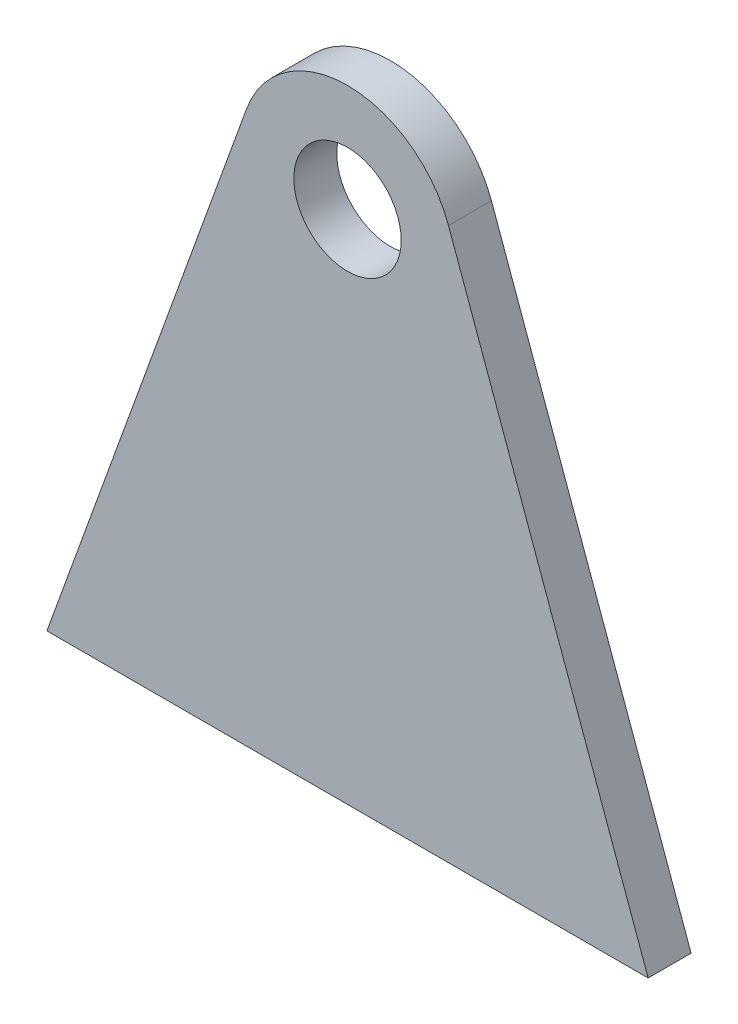
SolidWorks part; units mm, degrees
material "Plain Carbon Steel"
ref_plane "Front Plane" through (0, 0, 0) normal (0, 0, 1) x (1, 0, 0)
ref_plane "Top Plane" through (0, 0, 0) normal (0, 1, 0) x (1, 0, 0)
ref_plane "Right Plane" through (0, 0, 0) normal (1, 0, 0) x (0, 0, -1)
sketch "Lug Profile Sketch" plane through (0, 0, 0) normal (0, 0, 1) x (1, 0, 0)
  line L0 (-140, -240) -> (140, -240)
  line L1 (-47.0176, 17.0102) -> (-140, -240)
  line L2 (0, -11) -> (0, 11) construction
  line L3 (47.0176, 17.0102) -> (140, -240)
  circle A0 centre (0, 0) radius 25
  arc A1 (47.0176, 17.0102) -> (-47.0176, 17.0102) centre (0, 0) ccw
  point P6 (0, -240)
  dimension "D1" = 50
  dimension "D2" = 25
  dimension "D3" = 240
  dimension "D4" = 280
extrude "Lug Plate 20mm" add sketch "Lug Profile Sketch" along normal blind 20
